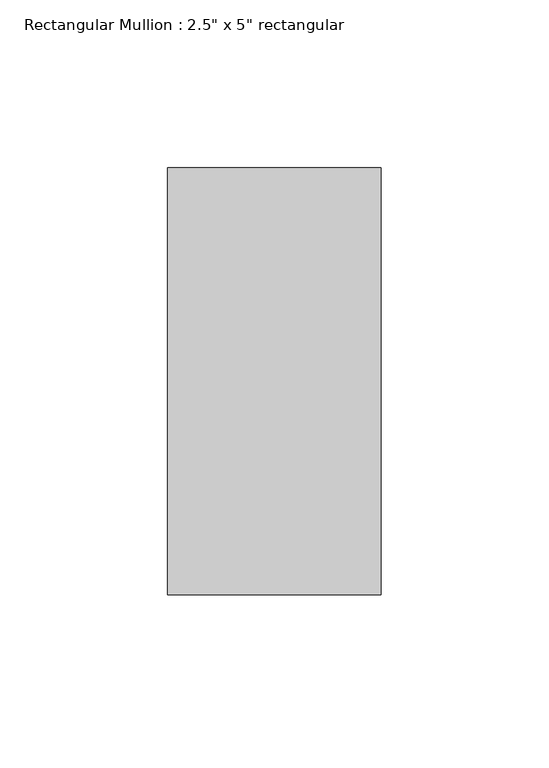
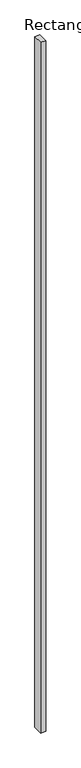
"""IFC4 building model written with IfcOpenShell, lengths in millimetres: member geometry."""

from ifc_helpers import new_model, si_unit, frame, origin, place, context, project, spatial, polyline, outline, extrude, source, transform, mapped, element, save


def member_8787ee90(model_context):
    return source(origin(), model_context, "Body", "SweptSolid", [
        extrude(outline(polyline([(0.0, 63.5), (0.0, -63.5), (-63.5, -63.5), (-63.5, 63.5), (0.0, 63.5)])), frame((0.0, 0.0, -9169.4), z_axis=(0.0, 0.0, 1.0), x_axis=(1.0, 0.0, 0.0)), (0.0, 0.0, 1.0), 9169.4),
    ])


if __name__ == "__main__":
    model = new_model("IFC4")
    model_context = context("Model", 3, world=origin())
    ifc_project = project(units=[si_unit("LENGTHUNIT", "METRE", prefix="MILLI")], contexts=[model_context])
    site = spatial("IfcSite", under=ifc_project)
    building = spatial("IfcBuilding", under=site)
    placement = place(None, origin())
    member_shape = member_8787ee90(model_context)
    element("IfcMember", 1, ObjectType="Rectangular Mullion : 2.5\" x 5\" rectangular", at=placement, inside=building, context=model_context, shape_type="MappedRepresentation", body=[
        mapped(member_shape, transform((0.0, 0.0, 0.0), x_axis=(1.0, 0.0, 0.0), y_axis=(0.0, 1.0, 0.0), z_axis=(0.0, 0.0, 1.0))),
    ])
    save(model, "model.ifc")

# Revit data of these elements
# Type "Rectangular Mullion : 2.5\" x 5\" rectangular"
#   built-in parameter 1007304 = 0.416667 (stored number, unit not read)
#   built-in parameter 1007301 = 0.104167 (stored number, unit not read)
#   built-in parameter 1007300 = 0.104167 (stored number, unit not read)
# Element 1 (IfcMember, "Rectangular Mullion : 2.5\" x 5\" rectangular")
#   Materials on its faces: "Aluminum"
# Materials
#   "Aluminum": class "Metal", colour RGB 247 247 247, transparency 0, Description = "Aluminum 6061", Cost = 0
